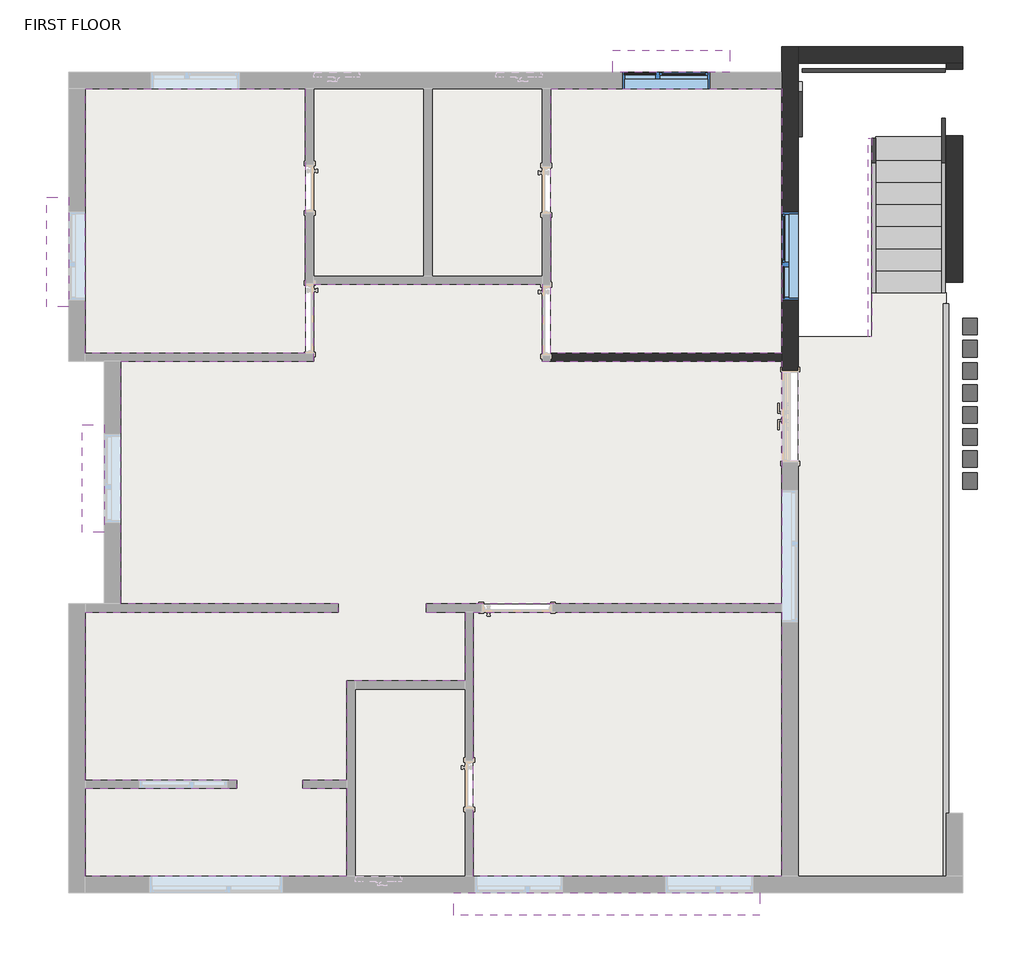
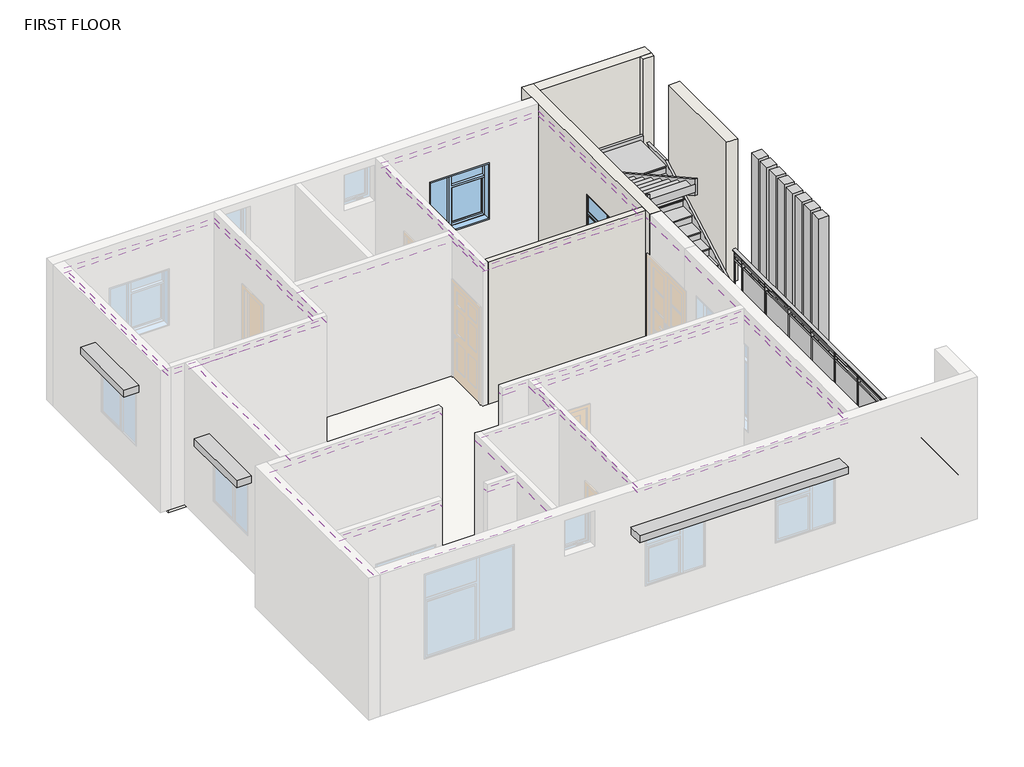
# One storey, part 2 of 2: 10 coverings, 5 members, 5 proxies, 4 walls, 2 slabs, 2 windows, 1 railing, 1 stair flight.
"""IFC4 building model written with IfcOpenShell, lengths in millimetres."""

from ifc_helpers import new_model, si_unit, point, frame, origin, place, context, project, spatial, polyline, ellipse_curve, trimmed, outline, extrude, faceted_brep, transform, mapped, element, save
from ifc_brep_helpers import plane_surface, extruded_surface, advanced_brep
from components import generic_models_10_generic_models_10_ac10314b, generic_models_3_generic_models_3_71021abf, generic_models_4_generic_models_4_4e8aec35, generic_models_7_generic_models_6_617e5b9e, generic_models_8_generic_models_8_43166a7e, stair_flight_d4afe6aa, window_casement_double_sidelight_window_4_x_4_2a492e8f

model = new_model("IFC4")

# Units and contexts
model_context = context("Model", 3, world=origin())
ifc_project = project(units=[si_unit("LENGTHUNIT", "METRE", prefix="MILLI")], contexts=[model_context])

# Site, building, storey
site = spatial("IfcSite", under=ifc_project)
building = spatial("IfcBuilding", under=site)
storey = spatial("IfcBuildingStorey", under=building, Name="FIRST FLOOR", Elevation=3048.0)

# Proxies
placement = place(None, origin())
generic_models_10_generic_models_10_shape = generic_models_10_generic_models_10_ac10314b(model_context)
element("IfcBuildingElementProxy", 1, Name="Generic Models 10 : Generic Models 10", ObjectType="Generic Models 10 : Generic Models 10", at=placement, inside=storey, context=model_context, shape_type="MappedRepresentation", body=[
    mapped(generic_models_10_generic_models_10_shape, transform((0.0, 0.0, 0.0), x_axis=(1.0, 0.0, 0.0), y_axis=(0.0, 1.0, 0.0), z_axis=(0.0, 0.0, 1.0))),
])
generic_models_3_generic_models_3_shape = generic_models_3_generic_models_3_71021abf(model_context)
element("IfcBuildingElementProxy", 2, Name="Generic Models 3 : Generic Models 3", ObjectType="Generic Models 3 : Generic Models 3", at=placement, inside=storey, context=model_context, shape_type="MappedRepresentation", body=[
    mapped(generic_models_3_generic_models_3_shape, transform((0.0, 0.0, 0.0), x_axis=(1.0, 0.0, 0.0), y_axis=(0.0, 1.0, 0.0), z_axis=(0.0, 0.0, 1.0))),
])
generic_models_4_generic_models_4_shape = generic_models_4_generic_models_4_4e8aec35(model_context)
element("IfcBuildingElementProxy", 3, Name="Generic Models 4 : Generic Models 4", ObjectType="Generic Models 4 : Generic Models 4", at=placement, inside=storey, context=model_context, shape_type="MappedRepresentation", body=[
    mapped(generic_models_4_generic_models_4_shape, transform((0.0, 0.0, 0.0), x_axis=(1.0, 0.0, 0.0), y_axis=(0.0, 1.0, 0.0), z_axis=(0.0, 0.0, 1.0))),
])
generic_models_7_generic_models_6_shape = generic_models_7_generic_models_6_617e5b9e(model_context)
element("IfcBuildingElementProxy", 4, Name="Generic Models 7 : Generic Models 6", ObjectType="Generic Models 7 : Generic Models 6", at=placement, inside=storey, context=model_context, shape_type="MappedRepresentation", body=[
    mapped(generic_models_7_generic_models_6_shape, transform((0.0, 0.0, 3048.0), x_axis=(1.0, 0.0, 0.0), y_axis=(0.0, 1.0, 0.0), z_axis=(0.0, 0.0, 1.0))),
])
generic_models_8_generic_models_8_shape = generic_models_8_generic_models_8_43166a7e(model_context)
element("IfcBuildingElementProxy", 5, Name="Generic Models 8 : Generic Models 8", ObjectType="Generic Models 8 : Generic Models 8", at=placement, inside=storey, context=model_context, shape_type="MappedRepresentation", body=[
    mapped(generic_models_8_generic_models_8_shape, transform((0.0, 0.0, 0.0), x_axis=(1.0, 0.0, 0.0), y_axis=(0.0, 1.0, 0.0), z_axis=(0.0, 0.0, 1.0))),
])

# Coverings
element("IfcCovering", 6, ObjectType="GWB on Mtl. Stud", at=placement, inside=storey, context=model_context, shape_type="SweptSolid", body=[
    extrude(outline(polyline([(-12301.4656154, -3057.0499125), (-14396.9656154, -3057.0499125), (-14396.9656154, -732.9499125), (-10895.4913348, -732.9499125), (-10895.4913348, -618.6499125), (-13901.6656154, -618.6499125), (-13901.6656154, 2734.1500875), (-11234.6656154, 2734.1500875), (-11234.6656154, 3800.9500875), (-8072.3656154, 3800.9500875), (-8072.3656154, 2734.1500875), (-4757.6656154, 2734.1500875), (-4757.6656154, 2581.7500875), (-4757.6656154, 1362.5500875), (-4757.6656154, -618.6499125), (-9676.2913348, -618.6499125), (-9676.2913348, -732.9499125), (-9139.1656154, -732.9499125), (-9139.1656154, -1685.4499125), (-10777.4656154, -1685.4499125), (-10777.4656154, -3057.0499125), (-11387.0656154, -3057.0499125), (-11387.0656154, -3171.3499125), (-10777.4656154, -3171.3499125), (-10777.4656154, -4390.5499125), (-14396.9656154, -4390.5499125), (-14396.9656154, -3171.3499125), (-12301.4656154, -3171.3499125), (-12301.4656154, -3057.0499125)])), frame((0.0, 0.0, 5943.6), z_axis=(0.0, 0.0, 1.0), x_axis=(1.0, 0.0, 0.0)), (0.0, 0.0, 1.0), 107.95),
])
element("IfcCovering", 7, ObjectType="GWB on Mtl. Stud", at=placement, inside=storey, context=model_context, shape_type="SweptSolid", body=[
    extrude(outline(polyline([(-12301.4656154, -3057.0499125), (-14396.9656154, -3057.0499125), (-14396.9656154, -732.9499125), (-10895.4913348, -732.9499125), (-10895.4913348, -618.6499125), (-13901.6656154, -618.6499125), (-13901.6656154, 2734.1500875), (-11234.6656154, 2734.1500875), (-11234.6656154, 3800.9500875), (-8072.3656154, 3800.9500875), (-8072.3656154, 2734.1500875), (-4757.6656154, 2734.1500875), (-4757.6656154, 2581.7500875), (-4757.6656154, 1362.5500875), (-4757.6656154, -618.6499125), (-9676.2913348, -618.6499125), (-9676.2913348, -732.9499125), (-9139.1656154, -732.9499125), (-9139.1656154, -1685.4499125), (-10777.4656154, -1685.4499125), (-10777.4656154, -3057.0499125), (-11387.0656154, -3057.0499125), (-11387.0656154, -3171.3499125), (-10777.4656154, -3171.3499125), (-10777.4656154, -4390.5499125), (-14396.9656154, -4390.5499125), (-14396.9656154, -3171.3499125), (-12301.4656154, -3171.3499125), (-12301.4656154, -3057.0499125)])), frame((0.0, 0.0, 5943.6), z_axis=(0.0, 0.0, 1.0), x_axis=(1.0, 0.0, 0.0)), (0.0, 0.0, 1.0), 107.95),
])
element("IfcCovering", 8, ObjectType="GWB on Mtl. Stud", at=placement, inside=storey, context=model_context, shape_type="SweptSolid", body=[
    extrude(outline(polyline([(-12301.4656154, -3057.0499125), (-14396.9656154, -3057.0499125), (-14396.9656154, -732.9499125), (-10895.4913348, -732.9499125), (-10895.4913348, -618.6499125), (-13901.6656154, -618.6499125), (-13901.6656154, 2734.1500875), (-11234.6656154, 2734.1500875), (-11234.6656154, 3800.9500875), (-8072.3656154, 3800.9500875), (-8072.3656154, 2734.1500875), (-4757.6656154, 2734.1500875), (-4757.6656154, 2581.7500875), (-4757.6656154, 1362.5500875), (-4757.6656154, -618.6499125), (-9676.2913348, -618.6499125), (-9676.2913348, -732.9499125), (-9139.1656154, -732.9499125), (-9139.1656154, -1685.4499125), (-10777.4656154, -1685.4499125), (-10777.4656154, -3057.0499125), (-11387.0656154, -3057.0499125), (-11387.0656154, -3171.3499125), (-10777.4656154, -3171.3499125), (-10777.4656154, -4390.5499125), (-14396.9656154, -4390.5499125), (-14396.9656154, -3171.3499125), (-12301.4656154, -3171.3499125), (-12301.4656154, -3057.0499125)])), frame((0.0, 0.0, 5943.6), z_axis=(0.0, 0.0, 1.0), x_axis=(1.0, 0.0, 0.0)), (0.0, 0.0, 1.0), 107.95),
])
element("IfcCovering", 9, ObjectType="recessed ceiling", at=placement, inside=storey, context=model_context, shape_type="SweptSolid", body=[
    extrude(outline(polyline([(-14396.9656154, 2848.4500875), (-14396.9656154, 6506.0500875), (-11348.9656154, 6506.0500875), (-11348.9656154, 2848.4500875), (-14396.9656154, 2848.4500875)])), frame((0.0, 0.0, 5943.6), z_axis=(0.0, 0.0, 1.0), x_axis=(1.0, 0.0, 0.0)), (0.0, 0.0, 1.0), 107.95),
])
element("IfcCovering", 10, ObjectType="recessed ceiling", at=placement, inside=storey, context=model_context, shape_type="SweptSolid", body=[
    extrude(outline(polyline([(-11348.9656154, 6506.0500875), (-11348.9656154, 2848.4500875), (-14396.9656154, 2848.4500875), (-14396.9656154, 6506.0500875), (-11348.9656154, 6506.0500875)]), holes=[polyline([(-11653.7656154, 6201.2500875), (-14092.1656154, 6201.2500875), (-14092.1656154, 3153.2500875), (-11653.7656154, 3153.2500875), (-11653.7656154, 6201.2500875)])]), frame((0.0, 0.0, 5842.0), z_axis=(0.0, 0.0, 1.0), x_axis=(1.0, 0.0, 0.0)), (0.0, 0.0, 1.0), 107.95),
])
element("IfcCovering", 11, ObjectType="recessed ceiling", at=placement, inside=storey, context=model_context, shape_type="SweptSolid", body=[
    extrude(outline(polyline([(-7958.0656154, 2848.4500875), (-7958.0656154, 6506.0500875), (-4757.6656154, 6506.0500875), (-4757.6656154, 2848.4500875), (-7958.0656154, 2848.4500875)])), frame((0.0, 0.0, 5943.6), z_axis=(0.0, 0.0, 1.0), x_axis=(1.0, 0.0, 0.0)), (0.0, 0.0, 1.0), 107.95),
])
element("IfcCovering", 12, ObjectType="recessed ceiling", at=placement, inside=storey, context=model_context, shape_type="SweptSolid", body=[
    extrude(outline(polyline([(-4757.6656154, 6506.0500875), (-4757.6656154, 2848.4500875), (-7958.0656154, 2848.4500875), (-7958.0656154, 6506.0500875), (-4757.6656154, 6506.0500875)]), holes=[polyline([(-5062.4656154, 6201.2500875), (-7653.2656154, 6201.2500875), (-7653.2656154, 3153.2500875), (-5062.4656154, 3153.2500875), (-5062.4656154, 6201.2500875)])]), frame((0.0, 0.0, 5842.0), z_axis=(0.0, 0.0, 1.0), x_axis=(1.0, 0.0, 0.0)), (0.0, 0.0, 1.0), 107.95),
])
element("IfcCovering", 13, ObjectType="recessed ceiling", at=placement, inside=storey, context=model_context, shape_type="SweptSolid", body=[
    extrude(outline(polyline([(-4757.6656154, -732.9499125), (-4757.6656154, -4390.5499125), (-9024.8656154, -4390.5499125), (-9024.8656154, -732.9499125), (-4757.6656154, -732.9499125)])), frame((0.0, 0.0, 5943.6), z_axis=(0.0, 0.0, 1.0), x_axis=(1.0, 0.0, 0.0)), (0.0, 0.0, 1.0), 107.95),
])
element("IfcCovering", 14, ObjectType="recessed ceiling", at=placement, inside=storey, context=model_context, shape_type="SweptSolid", body=[
    extrude(outline(polyline([(-4757.6656154, -732.9499125), (-4757.6656154, -4390.5499125), (-9024.8656154, -4390.5499125), (-9024.8656154, -732.9499125), (-4757.6656154, -732.9499125)])), frame((0.0, 0.0, 5943.6), z_axis=(0.0, 0.0, 1.0), x_axis=(1.0, 0.0, 0.0)), (0.0, 0.0, 1.0), 107.95),
])
element("IfcCovering", 15, ObjectType="recessed ceiling", at=placement, inside=storey, context=model_context, shape_type="SweptSolid", body=[
    extrude(outline(polyline([(-4757.6656154, -732.9499125), (-4757.6656154, -4390.5499125), (-9024.8656154, -4390.5499125), (-9024.8656154, -732.9499125), (-4757.6656154, -732.9499125)]), holes=[polyline([(-5062.4656154, -1037.7499125), (-8720.0656154, -1037.7499125), (-8720.0656154, -4085.7499125), (-5062.4656154, -4085.7499125), (-5062.4656154, -1037.7499125)])]), frame((0.0, 0.0, 5842.0), z_axis=(0.0, 0.0, 1.0), x_axis=(1.0, 0.0, 0.0)), (0.0, 0.0, 1.0), 107.95),
])

# Members
element("IfcMember", 16, ObjectType="Stringer - 2\" Width", at=placement, inside=storey, context=model_context, shape_type="SweptSolid", body=[
    extrude(outline(polyline([(3686.6500875, 3048.0), (3686.6500875, 3255.5983948), (5751.3729769, 4402.6666667), (5820.2500875, 4402.6666667), (5820.2500875, 4092.253054), (3940.5945903, 3048.0), (3686.6500875, 3048.0)])), frame((-3513.0656154, 0.0, 0.0), z_axis=(1.0, 0.0, 0.0), x_axis=(0.0, 1.0, 0.0)), (0.0, 0.0, 1.0), 50.8),
])
element("IfcMember", 17, ObjectType="Stringer - 2\" Width", at=placement, inside=storey, context=model_context, shape_type="SweptSolid", body=[
    extrude(outline(polyline([(5820.2500875, 4610.2650614), (5820.2500875, 4261.5863873), (3077.0500875, 5785.5863873), (3077.0500875, 6134.2650614), (5820.2500875, 4610.2650614)])), frame((-3563.8656154, 0.0, 0.0), z_axis=(1.0, 0.0, 0.0), x_axis=(0.0, 1.0, 0.0)), (0.0, 0.0, 1.0), 50.8),
])
element("IfcMember", 18, ObjectType="Stringer - 2\" Width", at=placement, inside=storey, context=model_context, shape_type="SweptSolid", body=[
    extrude(outline(polyline([(3686.6500875, 3048.0), (3686.6500875, 3255.5983948), (5888.5329769, 4478.8666667), (6516.1545903, 4478.8666667), (3940.5945903, 3048.0), (3686.6500875, 3048.0)])), frame((-2547.8656154, 0.0, 0.0), z_axis=(1.0, 0.0, 0.0), x_axis=(0.0, 1.0, 0.0)), (0.0, 0.0, 1.0), 50.8),
])
element("IfcMember", 19, ObjectType="Stringer - 2\" Width", at=placement, inside=storey, context=model_context, shape_type="SweptSolid", body=[
    extrude(outline(polyline([(-2497.0656154, 6785.4500875), (-2497.0656154, 6734.6500875), (-4478.2656154, 6734.6500875), (-4478.2656154, 6785.4500875), (-2497.0656154, 6785.4500875)])), frame((0.0, 0.0, 4174.0666667), z_axis=(0.0, 0.0, 1.0), x_axis=(1.0, 0.0, 0.0)), (0.0, 0.0, 1.0), 304.8),
])
element("IfcMember", 20, ObjectType="Stringer - 2\" Width", at=placement, inside=storey, context=model_context, shape_type="SweptSolid", body=[
    extrude(outline(polyline([(5977.7855847, 4174.0666667), (3077.0500875, 5785.5863873), (3077.0500875, 6134.2650614), (6605.4071981, 4174.0666667), (5977.7855847, 4174.0666667)])), frame((-4529.0656154, 0.0, 0.0), z_axis=(1.0, 0.0, 0.0), x_axis=(0.0, 1.0, 0.0)), (0.0, 0.0, 1.0), 50.8),
])

# Railing
element("IfcRailing", 21, ObjectType="Glass Panel - Bottom Fill", at=placement, inside=storey, context=model_context, shape_type="SolidModel", body=[
    advanced_brep(
    [(-2522.4656154, -4390.5499125, 3962.4), (-2446.2656154, -4390.5499125, 3962.4), (-2522.4656154, 3534.2500875, 3962.4), (-2446.2656154, 3534.2500875, 3962.4)],
    [
        (0, 1, ellipse_curve(frame((-2484.3656154, -4390.5499125, 3962.4), z_axis=(0.0, -1.0, 0.0), x_axis=(1.0, 0.0, 0.0)), 38.1, 28.575)),
        (1, 0, ellipse_curve(frame((-2484.3656154, -4390.5499125, 3962.4), z_axis=(0.0, -1.0, 0.0), x_axis=(1.0, 0.0, 0.0)), 38.1, 28.575)),
        (2, 3, ellipse_curve(frame((-2484.3656154, 3534.2500875, 3962.4), z_axis=(0.0, 1.0, 0.0), x_axis=(1.0, 0.0, 0.0)), 38.1, 28.575)),
        (3, 2, ellipse_curve(frame((-2484.3656154, 3534.2500875, 3962.4), z_axis=(0.0, 1.0, 0.0), x_axis=(1.0, 0.0, 0.0)), 38.1, 28.575)),
        (0, 2),
        (3, 1),
    ],
    [
        plane_surface(frame((-2484.3656154, -4390.5499125, 3962.4), z_axis=(0.0, -1.0, 0.0), x_axis=(0.0, 0.0, 1.0))),
        plane_surface(frame((-2484.3656154, 3534.2500875, 3962.4), z_axis=(0.0, 1.0, 0.0), x_axis=(0.0, 0.0, 1.0))),
        extruded_surface(trimmed(ellipse_curve(frame((-2484.3656154, 3534.2500875, 3962.4), z_axis=(0.0, -1.0, 0.0), x_axis=(1.0, 0.0, 0.0)), 38.1, 28.575), [point((-2522.4656154, 3534.2500875, 3962.4))], [point((-2446.2656154, 3534.2500875, 3962.4))], True, "CARTESIAN"), (0.0, -7924.799999999999, 0.0), 7924.799999999999),
        extruded_surface(trimmed(ellipse_curve(frame((-2484.3656154, 3534.2500875, 3962.4), z_axis=(0.0, -1.0, 0.0), x_axis=(1.0, 0.0, 0.0)), 38.1, 28.575), [point((-2446.2656154, 3534.2500875, 3962.4))], [point((-2522.4656154, 3534.2500875, 3962.4))], True, "CARTESIAN"), (0.0, -7924.799999999999, 0.0), 7924.799999999999),
    ],
    [
        (0, [[1, 2]]),
        (1, [[3, 4]]),
        (2, [[-1, 5, -4, 6]]),
        (3, [[-2, -6, -3, -5]]),
    ],
),
    extrude(outline(polyline([(-2471.6656154, -4390.5499125), (-2497.0656154, -4390.5499125), (-2497.0656154, 3534.2500875), (-2471.6656154, 3534.2500875), (-2471.6656154, -4390.5499125)])), frame((0.0, 0.0, 3848.1), z_axis=(0.0, 0.0, 1.0), x_axis=(1.0, 0.0, 0.0)), (0.0, 0.0, 1.0), 25.4),
    extrude(outline(polyline([(-2471.6656154, -4390.5499125), (-2497.0656154, -4390.5499125), (-2497.0656154, 3534.2500875), (-2471.6656154, 3534.2500875), (-2471.6656154, -4390.5499125)])), frame((0.0, 0.0, 3746.5), z_axis=(0.0, 0.0, 1.0), x_axis=(1.0, 0.0, 0.0)), (0.0, 0.0, 1.0), 25.4),
    extrude(outline(polyline([(-2458.9656154, 3223.1000875), (-2509.7656154, 3223.1000875), (-2509.7656154, 3235.8000875), (-2458.9656154, 3235.8000875), (-2458.9656154, 3223.1000875)])), frame((0.0, 0.0, 3048.0), z_axis=(0.0, 0.0, 1.0), x_axis=(1.0, 0.0, 0.0)), (0.0, 0.0, 1.0), 885.825),
    extrude(outline(polyline([(-2490.9007724, 2416.6500875), (-2490.9007724, 3229.4500875), (-2484.5507724, 3229.4500875), (-2484.5507724, 2416.6500875), (-2490.9007724, 2416.6500875)])), frame((0.0, 0.0, 3149.6), z_axis=(0.0, 0.0, 1.0), x_axis=(1.0, 0.0, 0.0)), (0.0, 0.0, 1.0), 596.9),
    extrude(outline(polyline([(-2458.9656154, 2410.3000875), (-2509.7656154, 2410.3000875), (-2509.7656154, 2423.0000875), (-2458.9656154, 2423.0000875), (-2458.9656154, 2410.3000875)])), frame((0.0, 0.0, 3048.0), z_axis=(0.0, 0.0, 1.0), x_axis=(1.0, 0.0, 0.0)), (0.0, 0.0, 1.0), 885.825),
    extrude(outline(polyline([(-2490.9007724, 1603.8500875), (-2490.9007724, 2416.6500875), (-2484.5507724, 2416.6500875), (-2484.5507724, 1603.8500875), (-2490.9007724, 1603.8500875)])), frame((0.0, 0.0, 3149.6), z_axis=(0.0, 0.0, 1.0), x_axis=(1.0, 0.0, 0.0)), (0.0, 0.0, 1.0), 596.9),
    extrude(outline(polyline([(-2458.9656154, 1597.5000875), (-2509.7656154, 1597.5000875), (-2509.7656154, 1610.2000875), (-2458.9656154, 1610.2000875), (-2458.9656154, 1597.5000875)])), frame((0.0, 0.0, 3048.0), z_axis=(0.0, 0.0, 1.0), x_axis=(1.0, 0.0, 0.0)), (0.0, 0.0, 1.0), 885.825),
    extrude(outline(polyline([(-2490.9007724, 791.0500875), (-2490.9007724, 1603.8500875), (-2484.5507724, 1603.8500875), (-2484.5507724, 791.0500875), (-2490.9007724, 791.0500875)])), frame((0.0, 0.0, 3149.6), z_axis=(0.0, 0.0, 1.0), x_axis=(1.0, 0.0, 0.0)), (0.0, 0.0, 1.0), 596.9),
    extrude(outline(polyline([(-2458.9656154, 784.7000875), (-2509.7656154, 784.7000875), (-2509.7656154, 797.4000875), (-2458.9656154, 797.4000875), (-2458.9656154, 784.7000875)])), frame((0.0, 0.0, 3048.0), z_axis=(0.0, 0.0, 1.0), x_axis=(1.0, 0.0, 0.0)), (0.0, 0.0, 1.0), 885.825),
    extrude(outline(polyline([(-2490.9007724, -21.7499125), (-2490.9007724, 791.0500875), (-2484.5507724, 791.0500875), (-2484.5507724, -21.7499125), (-2490.9007724, -21.7499125)])), frame((0.0, 0.0, 3149.6), z_axis=(0.0, 0.0, 1.0), x_axis=(1.0, 0.0, 0.0)), (0.0, 0.0, 1.0), 596.9),
    extrude(outline(polyline([(-2458.9656154, -28.0999125), (-2509.7656154, -28.0999125), (-2509.7656154, -15.3999125), (-2458.9656154, -15.3999125), (-2458.9656154, -28.0999125)])), frame((0.0, 0.0, 3048.0), z_axis=(0.0, 0.0, 1.0), x_axis=(1.0, 0.0, 0.0)), (0.0, 0.0, 1.0), 885.825),
    extrude(outline(polyline([(-2490.9007724, -834.5499125), (-2490.9007724, -21.7499125), (-2484.5507724, -21.7499125), (-2484.5507724, -834.5499125), (-2490.9007724, -834.5499125)])), frame((0.0, 0.0, 3149.6), z_axis=(0.0, 0.0, 1.0), x_axis=(1.0, 0.0, 0.0)), (0.0, 0.0, 1.0), 596.9),
    extrude(outline(polyline([(-2458.9656154, -840.8999125), (-2509.7656154, -840.8999125), (-2509.7656154, -828.1999125), (-2458.9656154, -828.1999125), (-2458.9656154, -840.8999125)])), frame((0.0, 0.0, 3048.0), z_axis=(0.0, 0.0, 1.0), x_axis=(1.0, 0.0, 0.0)), (0.0, 0.0, 1.0), 885.825),
    extrude(outline(polyline([(-2490.9007724, -1647.3499125), (-2490.9007724, -834.5499125), (-2484.5507724, -834.5499125), (-2484.5507724, -1647.3499125), (-2490.9007724, -1647.3499125)])), frame((0.0, 0.0, 3149.6), z_axis=(0.0, 0.0, 1.0), x_axis=(1.0, 0.0, 0.0)), (0.0, 0.0, 1.0), 596.9),
    extrude(outline(polyline([(-2458.9656154, -1653.6999125), (-2509.7656154, -1653.6999125), (-2509.7656154, -1640.9999125), (-2458.9656154, -1640.9999125), (-2458.9656154, -1653.6999125)])), frame((0.0, 0.0, 3048.0), z_axis=(0.0, 0.0, 1.0), x_axis=(1.0, 0.0, 0.0)), (0.0, 0.0, 1.0), 885.825),
    extrude(outline(polyline([(-2490.9007724, -2460.1499125), (-2490.9007724, -1647.3499125), (-2484.5507724, -1647.3499125), (-2484.5507724, -2460.1499125), (-2490.9007724, -2460.1499125)])), frame((0.0, 0.0, 3149.6), z_axis=(0.0, 0.0, 1.0), x_axis=(1.0, 0.0, 0.0)), (0.0, 0.0, 1.0), 596.9),
    extrude(outline(polyline([(-2458.9656154, -2466.4999125), (-2509.7656154, -2466.4999125), (-2509.7656154, -2453.7999125), (-2458.9656154, -2453.7999125), (-2458.9656154, -2466.4999125)])), frame((0.0, 0.0, 3048.0), z_axis=(0.0, 0.0, 1.0), x_axis=(1.0, 0.0, 0.0)), (0.0, 0.0, 1.0), 885.825),
    extrude(outline(polyline([(-2490.9007724, -3272.9499125), (-2490.9007724, -2460.1499125), (-2484.5507724, -2460.1499125), (-2484.5507724, -3272.9499125), (-2490.9007724, -3272.9499125)])), frame((0.0, 0.0, 3149.6), z_axis=(0.0, 0.0, 1.0), x_axis=(1.0, 0.0, 0.0)), (0.0, 0.0, 1.0), 596.9),
    extrude(outline(polyline([(-2458.9656154, -3279.2999125), (-2509.7656154, -3279.2999125), (-2509.7656154, -3266.5999125), (-2458.9656154, -3266.5999125), (-2458.9656154, -3279.2999125)])), frame((0.0, 0.0, 3048.0), z_axis=(0.0, 0.0, 1.0), x_axis=(1.0, 0.0, 0.0)), (0.0, 0.0, 1.0), 885.825),
    extrude(outline(polyline([(-2490.9007724, -4085.7499125), (-2490.9007724, -3272.9499125), (-2484.5507724, -3272.9499125), (-2484.5507724, -4085.7499125), (-2490.9007724, -4085.7499125)])), frame((0.0, 0.0, 3149.6), z_axis=(0.0, 0.0, 1.0), x_axis=(1.0, 0.0, 0.0)), (0.0, 0.0, 1.0), 596.9),
    extrude(outline(polyline([(-2458.9656154, -4092.0999125), (-2509.7656154, -4092.0999125), (-2509.7656154, -4079.3999125), (-2458.9656154, -4079.3999125), (-2458.9656154, -4092.0999125)])), frame((0.0, 0.0, 3048.0), z_axis=(0.0, 0.0, 1.0), x_axis=(1.0, 0.0, 0.0)), (0.0, 0.0, 1.0), 885.825),
    extrude(outline(polyline([(-2474.8406154, 3521.5500875), (-2493.8906154, 3521.5500875), (-2493.8906154, 3540.6000875), (-2474.8406154, 3540.6000875), (-2474.8406154, 3521.5500875)])), frame((0.0, 0.0, 3048.0), z_axis=(0.0, 0.0, 1.0), x_axis=(1.0, 0.0, 0.0)), (0.0, 0.0, 1.0), 885.825),
    extrude(outline(polyline([(-2474.8406154, -4396.8999125), (-2493.8906154, -4396.8999125), (-2493.8906154, -4377.8499125), (-2474.8406154, -4377.8499125), (-2474.8406154, -4396.8999125)])), frame((0.0, 0.0, 3048.0), z_axis=(0.0, 0.0, 1.0), x_axis=(1.0, 0.0, 0.0)), (0.0, 0.0, 1.0), 885.825),
])

# Slabs
element("IfcSlab", 22, at=placement, inside=storey, context=model_context, shape_type="SweptSolid", body=[
    extrude(outline(polyline([(-9710.6656154, 6506.0500875), (-9710.6656154, 3915.2500875), (-11234.6656154, 3915.2500875), (-11234.6656154, 6506.0500875), (-9710.6656154, 6506.0500875)])), frame((0.0, 0.0, 2895.6), z_axis=(0.0, 0.0, 1.0), x_axis=(1.0, 0.0, 0.0)), (0.0, 0.0, 1.0), 152.4),
    extrude(outline(polyline([(-8072.3656154, 6506.0500875), (-8072.3656154, 3915.2500875), (-9596.3656154, 3915.2500875), (-9596.3656154, 6506.0500875), (-8072.3656154, 6506.0500875)])), frame((0.0, 0.0, 2895.6), z_axis=(0.0, 0.0, 1.0), x_axis=(1.0, 0.0, 0.0)), (0.0, 0.0, 1.0), 152.4),
    extrude(outline(polyline([(-9139.1656154, -1799.7499125), (-9139.1656154, -4390.5499125), (-10663.1656154, -4390.5499125), (-10663.1656154, -1799.7499125), (-9139.1656154, -1799.7499125)])), frame((0.0, 0.0, 2895.6), z_axis=(0.0, 0.0, 1.0), x_axis=(1.0, 0.0, 0.0)), (0.0, 0.0, 1.0), 152.4),
])
element("IfcSlab", 23, ObjectType="ROSE MARBLE FLOOR", at=placement, inside=storey, context=model_context, shape_type="SweptSolid", body=[
    extrude(outline(polyline([(-11348.9656154, 6506.0500875), (-11348.9656154, 2848.4500875), (-14396.9656154, 2848.4500875), (-14396.9656154, 6506.0500875), (-11348.9656154, 6506.0500875)])), frame((0.0, 0.0, 2895.6), z_axis=(0.0, 0.0, 1.0), x_axis=(1.0, 0.0, 0.0)), (0.0, 0.0, 1.0), 152.4),
    extrude(outline(polyline([(-4757.6656154, 6506.0500875), (-4757.6656154, 2848.4500875), (-7958.0656154, 2848.4500875), (-7958.0656154, 6506.0500875), (-4757.6656154, 6506.0500875)])), frame((0.0, 0.0, 2895.6), z_axis=(0.0, 0.0, 1.0), x_axis=(1.0, 0.0, 0.0)), (0.0, 0.0, 1.0), 152.4),
    extrude(outline(polyline([(-13901.6656154, -618.6499125), (-13901.6656154, 2734.1500875), (-11234.6656154, 2734.1500875), (-11234.6656154, 3800.9500875), (-8072.3656154, 3800.9500875), (-8072.3656154, 2734.1500875), (-4757.6656154, 2734.1500875), (-4757.6656154, -618.6499125), (-9676.2913348, -618.6499125), (-9676.2913348, -732.9499125), (-9139.1656154, -732.9499125), (-9139.1656154, -1685.4499125), (-10777.4656154, -1685.4499125), (-10777.4656154, -3057.0499125), (-11387.0656154, -3057.0499125), (-11387.0656154, -3171.3499125), (-10777.4656154, -3171.3499125), (-10777.4656154, -4390.5499125), (-14396.9656154, -4390.5499125), (-14396.9656154, -3171.3499125), (-12301.4656154, -3171.3499125), (-12301.4656154, -3057.0499125), (-14396.9656154, -3057.0499125), (-14396.9656154, -732.9499125), (-10895.4913348, -732.9499125), (-10895.4913348, -618.6499125), (-13901.6656154, -618.6499125)])), frame((0.0, 0.0, 2895.6), z_axis=(0.0, 0.0, 1.0), x_axis=(1.0, 0.0, 0.0)), (0.0, 0.0, 1.0), 152.4),
    extrude(outline(polyline([(-4757.6656154, -4390.5499125), (-9024.8656154, -4390.5499125), (-9024.8656154, -732.9499125), (-4757.6656154, -732.9499125), (-4757.6656154, -4390.5499125)])), frame((0.0, 0.0, 2895.6), z_axis=(0.0, 0.0, 1.0), x_axis=(1.0, 0.0, 0.0)), (0.0, 0.0, 1.0), 152.4),
    extrude(outline(polyline([(-4529.0656154, 3051.6500875), (-4529.0656154, 3077.0500875), (-3513.0656154, 3077.0500875), (-3513.0656154, 3686.6500875), (-2484.3656154, 3686.6500875), (-2484.3656154, 3051.6500875), (-2484.3656154, -4390.5499125), (-4529.0656154, -4390.5499125), (-4529.0656154, 3051.6500875)])), frame((0.0, 0.0, 2895.6), z_axis=(0.0, 0.0, 1.0), x_axis=(1.0, 0.0, 0.0)), (0.0, 0.0, 1.0), 152.4),
])

# Stair flight
stair_flight_shape = stair_flight_d4afe6aa(model_context)
element("IfcStairFlight", 24, ObjectType="2\" Tread 1\" Nosing 1/4\" Riser", at=placement, inside=storey, context=model_context, shape_type="MappedRepresentation", body=[
    mapped(stair_flight_shape, transform((0.0, 0.0, 0.0), x_axis=(1.0, 0.0, 0.0), y_axis=(0.0, 1.0, 0.0), z_axis=(0.0, 0.0, 1.0))),
])

# Walls
element("IfcWall", 25, at=placement, inside=storey, context=model_context, shape_type="Brep", body=[
    faceted_brep([(-4529.0656154, 7090.2500875, 6096.0), (-4529.0656154, 6861.6500875, 6096.0), (-4529.0656154, 2581.7500875, 6096.0), (-4529.0656154, 2581.7500875, 5181.6), (-4529.0656154, 2607.1500875, 5181.6), (-4529.0656154, 2607.1500875, 3048.0), (-4529.0656154, 6861.6500875, 3048.0), (-4529.0656154, 7090.2500875, 3048.0), (-4529.0656154, 4803.1295492, 5181.6), (-4529.0656154, 4803.1295492, 3962.4), (-4529.0656154, 3583.9295492, 3962.4), (-4529.0656154, 3583.9295492, 5181.6), (-4757.6656154, 2581.7500875, 6096.0), (-4757.6656154, 2734.1500875, 6096.0), (-4757.6656154, 2848.4500875, 6096.0), (-4757.6656154, 6506.0500875, 6096.0), (-4757.6656154, 6734.6500875, 6096.0), (-4757.6656154, 7090.2500875, 6096.0), (-4757.6656154, 7090.2500875, 3048.0), (-4757.6656154, 6734.6500875, 3048.0), (-4757.6656154, 6506.0500875, 3048.0), (-4757.6656154, 2848.4500875, 3048.0), (-4757.6656154, 2734.1500875, 3048.0), (-4757.6656154, 2607.1500875, 3048.0), (-4757.6656154, 2607.1500875, 5181.6), (-4757.6656154, 2581.7500875, 5181.6), (-4757.6656154, 4803.1295492, 5181.6), (-4757.6656154, 3583.9295492, 5181.6), (-4757.6656154, 3583.9295492, 3962.4), (-4757.6656154, 4803.1295492, 3962.4)], [[[0, 1, 2, 3, 4, 5, 6, 7], [8, 9, 10, 11]], [[12, 13, 14, 15, 16, 17, 18, 19, 20, 21, 22, 23, 24, 25], [26, 27, 28, 29]], [[18, 7, 6, 5, 23, 22, 21, 20, 19]], [[2, 1, 0, 17, 16, 15, 14, 13, 12]], [[2, 12, 25, 3]], [[4, 24, 23, 5]], [[24, 4, 3, 25]], [[9, 8, 26, 29]], [[10, 9, 29, 28]], [[11, 10, 28, 27]], [[8, 11, 27, 26]], [[0, 7, 18, 17]]]),
])
element("IfcWall", 26, at=placement, inside=storey, context=model_context, shape_type="Brep", body=[
    faceted_brep([(-4757.6656154, 2848.4500875, 3048.0), (-7958.0656154, 2848.4500875, 3048.0), (-7958.0656154, 2848.4500875, 6096.0), (-4757.6656154, 2848.4500875, 6096.0), (-4757.6656154, 2734.1500875, 3048.0), (-4757.6656154, 2734.1500875, 6096.0), (-7958.0656154, 2734.1500875, 6096.0), (-7958.0656154, 2734.1500875, 3048.0), (-7958.0656154, 2816.7000875, 3048.0)], [[[0, 1, 2, 3]], [[4, 5, 6, 7]], [[1, 0, 4, 7, 8]], [[3, 2, 6, 5]], [[2, 1, 8, 7, 6]], [[0, 3, 5, 4]]]),
])
element("IfcWall", 27, at=placement, inside=storey, context=model_context, shape_type="Brep", body=[
    faceted_brep([(-4529.0656154, 6861.6500875, 3048.0), (-2484.7352148, 6861.6500875, 3048.0), (-2256.1352148, 6861.6500875, 3048.0), (-2256.1352148, 6861.6500875, 6096.0), (-2484.7352148, 6861.6500875, 6096.0), (-4529.0656154, 6861.6500875, 6096.0), (-4529.0656154, 7090.2500875, 3048.0), (-4529.0656154, 7090.2500875, 6096.0), (-2256.1352148, 7090.2500875, 6096.0), (-2256.1352148, 7090.2500875, 3048.0)], [[[0, 1, 2, 3, 4, 5]], [[6, 7, 8, 9]], [[2, 1, 0, 6, 9]], [[5, 4, 3, 8, 7]], [[0, 5, 7, 6]], [[3, 2, 9, 8]]]),
])
element("IfcWall", 28, at=placement, inside=storey, context=model_context, shape_type="SweptSolid", body=[
    extrude(outline(polyline([(-2256.1352148, 3826.3500875), (-2484.7352148, 3826.3500875), (-2484.7352148, 5858.3500875), (-2256.1352148, 5858.3500875), (-2256.1352148, 3826.3500875)])), frame((0.0, 0.0, 3048.0), z_axis=(0.0, 0.0, 1.0), x_axis=(1.0, 0.0, 0.0)), (0.0, 0.0, 1.0), 3048.0),
    extrude(outline(polyline([(-2484.7352148, 6861.6500875), (-2256.1352148, 6861.6500875), (-2256.1352148, 6772.7500875), (-2484.7352148, 6772.7500875), (-2484.7352148, 6861.6500875)])), frame((0.0, 0.0, 3048.0), z_axis=(0.0, 0.0, 1.0), x_axis=(1.0, 0.0, 0.0)), (0.0, 0.0, 1.0), 3048.0),
])

# Windows
window_casement_double_sidelight_window_4_x_4_shape = window_casement_double_sidelight_window_4_x_4_2a492e8f(model_context)
element("IfcWindow", 29, ObjectType="Window-Casement-Double-Sidelight : window 4' x 4'", at=placement, inside=storey, context=model_context, shape_type="MappedRepresentation", body=[
    mapped(window_casement_double_sidelight_window_4_x_4_shape, transform((-6357.8656154, 6620.3500875, 3048.0), x_axis=(1.0, 0.0, 0.0), y_axis=(0.0, 1.0, 0.0), z_axis=(0.0, 0.0, 1.0))),
])
element("IfcWindow", 30, ObjectType="Window-Casement-Double-Sidelight : window 4' x 4'", at=placement, inside=storey, context=model_context, shape_type="MappedRepresentation", body=[
    mapped(window_casement_double_sidelight_window_4_x_4_shape, transform((-4643.3656154, 4193.5295492, 3048.0), x_axis=(0.0, 1.0, 0.0), y_axis=(-1.0, 0.0, 0.0), z_axis=(0.0, 0.0, 1.0))),
])

save(model, "model.ifc")

# Revit data of these elements
# Type "GWB on Mtl. Stud"
#   Assembly Code = "C3030220"
#   built-in parameter 1002203 = 1 (stored number, unit not read)
#   built-in parameter 1002202 = 1 (stored number, unit not read)
#   Layers, outside or top first: 0' - 3 5/8" "Metal Stud Layer" (function 1); 0' - 0 5/8" "Gypsum Wall Board" (function 5)
# Type "recessed ceiling"
#   Assembly Code = "C3030220"
#   built-in parameter 1002203 = 1 (stored number, unit not read)
#   built-in parameter 1002202 = 1 (stored number, unit not read)
#   Layers, outside or top first: 0' - 3 5/8" "recessed ceiling" (function 1); 0' - 0 5/8" "LIGHT BEIGE" (function 5)
# Type "Glass Panel - Bottom Fill"
#   Assembly Code = "C2010400"
#   built-in parameter 1008612 = 0.0416667 (stored number, unit not read)
#   built-in parameter 1008611 = 0.0416667 (stored number, unit not read)
#   built-in parameter 1008609 = 0.333333 (stored number, unit not read)
#   built-in parameter 1008604 = 0.166667 (stored number, unit not read)
#   built-in parameter 1008603 = 0.166667 (stored number, unit not read)
#   Railing Height = 3' - 0"
#   built-in parameter 1008630 = 2
#   built-in parameter 1008610 = 2
#   built-in parameter 1008618 = Baluster - Square : 3/4"
# Type
#   Assembly Code = "B1010"
#   Function = 0
# Type "ROSE MARBLE FLOOR"
#   Assembly Code = "B1010"
#   Function = 0
#   Layers, outside or top first: 0' - 6" "MARBLE FLOORING" (function 1)
# Type
#   Assembly Code = "B2010"
#   Layers, outside or top first: 0' - 9" "LIGHT BEIGE" (function 1)
# Type
#   Assembly Code = "B2010"
#   Layers, outside or top first: 0' - 4 1/2" "LIGHT BEIGE" (function 1)
# Type "Window-Casement-Double-Sidelight : window 4' x 4'"
#   Type Mark = "22"
#   Fire Rating = "0.5h"
#   Assembly Code = "B2020100"
#   Analytic Construction = "Double glazing - domestic"
#   Window Inset [instance default] = 0' - 0 5/8"
#   Wall Thickness [instance default] = 0' - 6"
#   Visual Light Transmittance = 0.81
#   Transom Height Ratio = 0.3
#   Transom Height = 1' - 2.4"
#   Thermal Resistance (R) = 1.8146 (h·ft²·°F)/BTU
#   Solar Heat Gain Coefficient = 0.76
#   Side Width = 1' - 7.2"
#   Rough Width = 4' - 0 1/2"
#   Rough Height = 4' - 0 1/2"
#   Opening Window Width = 2' - 4.8"
#   Opening Window Height = 2' - 9.6"
#   Heat Transfer Coefficient (U) = 0.5511 BTU/(h·ft²·°F)
#   Height = 4' - 0"
#   Frame Gap 3 [instance default] = 0' - 1 83/128"
#   Frame Gap 2 [instance default] = 0' - 0 5/8"
#   Frame Gap 1 = 0' - 1 51/128"
#   Default Sill Height = 3' - 0"
#   Width = 4' - 0"
#   Frame Material = Metal - Aluminum
#   Glass Panel Material = Glass
#   Wall Closure = (empty or 0)
# Element 1 (IfcBuildingElementProxy, "Generic Models 10 : Generic Models 10")
#   Phase Created = New Construction
#   Materials on its faces: "LIGHT BEIGE"
# Element 2 (IfcBuildingElementProxy, "Generic Models 3 : Generic Models 3")
#   Phase Created = New Construction
#   Materials on its faces: "LIGHT BEIGE"
# Element 3 (IfcBuildingElementProxy, "Generic Models 4 : Generic Models 4")
#   Phase Created = New Construction
#   Materials on its faces: "LIGHT BEIGE"
# Element 4 (IfcBuildingElementProxy, "Generic Models 7 : Generic Models 6")
#   Phase Created = New Construction
#   Materials on its faces: "LIGHT BEIGE"
# Element 5 (IfcBuildingElementProxy, "Generic Models 8 : Generic Models 8")
#   Phase Created = New Construction
#   Materials on its faces: "LIGHT BEIGE"
# Elements 6, 7, 8 (IfcCovering, "GWB on Mtl. Stud")
#   Height Offset From Level = 9' - 6"
#   Phase Created = New Construction
#   Materials on its faces: "Gypsum Wall Board", "Metal Stud Layer"
# Elements 9, 11, 13, 14 (IfcCovering, "recessed ceiling")
#   Height Offset From Level = 9' - 6"
#   Phase Created = New Construction
#   Materials on its faces: "LIGHT BEIGE", "recessed ceiling"
# Elements 10, 12, 15 (IfcCovering, "recessed ceiling")
#   Height Offset From Level = 9' - 2"
#   Phase Created = New Construction
#   Materials on its faces: "LIGHT BEIGE", "recessed ceiling"
# Elements 16, 17, 18, 19, 20 (IfcMember, "Stringer - 2\" Width")
#   Phase Created = New Construction
# Element 21 (IfcRailing, "Glass Panel - Bottom Fill")
#   Phase Created = New Construction
#   Materials on its faces: "Glass"
# Element 22 (IfcSlab)
#   Height Offset From Level = 0' - 0"
#   Phase Created = New Construction
# Element 23 (IfcSlab, "ROSE MARBLE FLOOR")
#   Height Offset From Level = 0' - 0"
#   Phase Created = New Construction
#   Materials on its faces: "MARBLE FLOORING"
# Element 24 (IfcStairFlight, "2\" Tread 1\" Nosing 1/4\" Riser")
#   Phase Created = New Construction
# Elements 25, 26, 27, 28 (IfcWall)
#   Top Offset = 0' - 0"
#   Base Offset = 0' - 0"
#   wall height = 10' - 0"
#   Phase Created = New Construction
#   Base Constraint = FIRST FLOOR
#   Top Constraint = SECOND FLR
#   Materials on its faces: "LIGHT BEIGE"
# Element 29 (IfcWindow, "Window-Casement-Double-Sidelight : window 4' x 4'")
#   Mark = "23"
#   Window Inset = 0' - 0 5/8"
#   Frame Gap 3 = 0' - 1 83/128"
#   Frame Gap 2 = 0' - 0 5/8"
#   Phase Created = New Construction
#   Materials on its faces: "Metal - Aluminum", "Glass"
# Element 30 (IfcWindow, "Window-Casement-Double-Sidelight : window 4' x 4'")
#   Mark = "26"
#   Window Inset = 0' - 0 5/8"
#   Frame Gap 3 = 0' - 1 83/128"
#   Frame Gap 2 = 0' - 0 5/8"
#   Phase Created = New Construction
#   Materials on its faces: "Metal - Aluminum", "Glass"
# Materials
#   "Metal Stud Layer": class "Metal", colour RGB 199 199 199, transparency 0, Description = "Light gauge steel framing, thermal air layer", Cost = 0
#   "Gypsum Wall Board": class "Generic", colour RGB 127 127 127, transparency 0, Description = "Gypsum Wall Board", Cost = 0
#   "recessed ceiling": class "Generic", colour RGB 120 120 120, transparency 0, Cost = 0
#   "LIGHT BEIGE": class "Generic", colour RGB 120 120 120, transparency 0, Cost = 0
#   "MARBLE FLOORING": class "Generic", colour RGB 120 120 120, transparency 0, Cost = 0
#   "Metal - Aluminum": class "Metal", colour RGB 247 247 247, transparency 0
#   "Glass": class "Glass", colour RGB 0 128 192, transparency 0.75, Description = "Soda Lime Glass", Cost = 0
